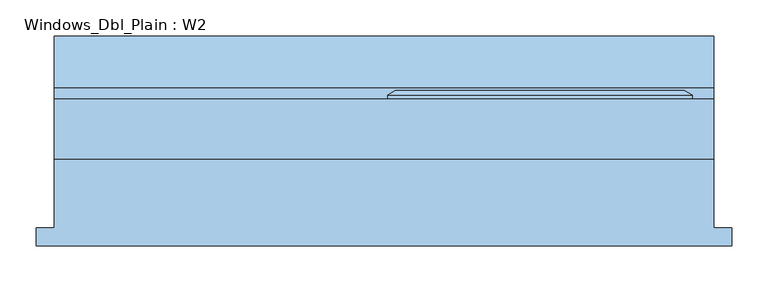
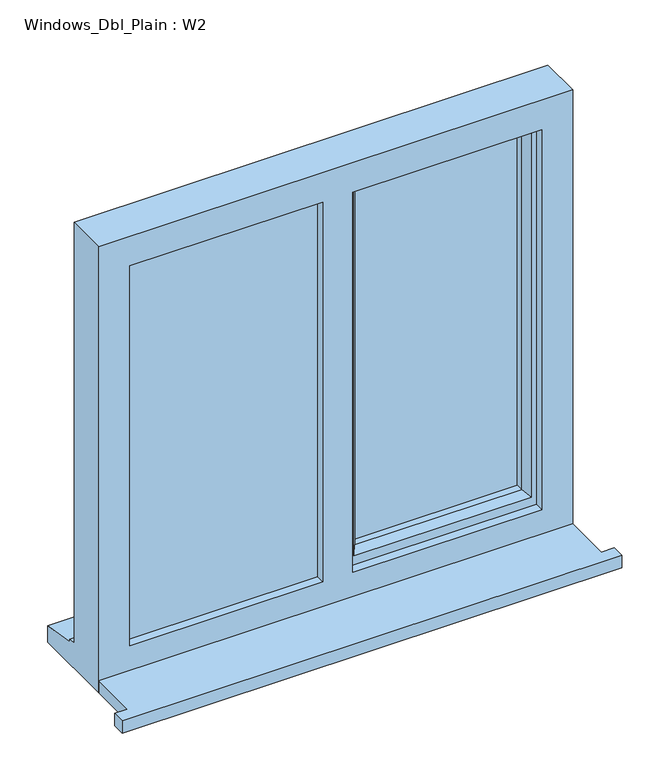
"""IFC4 building model written with IfcOpenShell, lengths in millimetres: window geometry, Windows_Dbl_Plain : W2."""

from ifc_helpers import new_model, si_unit, frame, origin, place, context, project, spatial, polyline, outline, extrude, faceted_brep, source, transform, mapped, element, save


def windows_dbl_plain_w2_c69f14ef(model_context):
    return source(origin(), model_context, "Body", "SolidModel", [
        extrude(outline(polyline([(-767.2, -130.8434322), (-767.2, -105.8434322), (-742.2, -105.8434322), (-742.2, -10.2434322), (172.2, -10.2434322), (172.2, -105.8434322), (197.2, -105.8434322), (197.2, -130.8434322), (-767.2, -130.8434322)])), frame((0.0, 0.0, 1200.0), z_axis=(0.0, 0.0, 1.0), x_axis=(1.0, 0.0, 0.0)), (0.0, 0.0, 1.0), 25.0),
        faceted_brep([(-280.0, 72.7565678, 2080.0), (-280.0, 78.5300705, 2080.0), (-280.0, 78.5300705, 1253.0), (-280.0, 72.7565678, 1253.0), (-270.0, 7.7565678, 2070.0), (-270.0, 72.7565678, 2070.0), (-270.0, 72.7565678, 1263.0), (-270.0, 7.7565678, 1263.0), (-230.0, 22.2494677, 2030.0), (-240.1480377, 7.7565678, 2040.1480377), (-240.1480377, 7.7565678, 1292.8519623), (-230.0, 22.2494677, 1303.0), (-230.0, 36.7565678, 2030.0), (-230.0, 36.7565678, 1303.0), (-240.0, 60.7565678, 2040.0), (-240.0, 36.7565678, 2040.0), (-240.0, 36.7565678, 1293.0), (-240.0, 60.7565678, 1293.0), (-230.0, 78.5300705, 2030.0), (-230.0, 60.7565678, 2030.0), (-230.0, 60.7565678, 1303.0), (-230.0, 78.5300705, 1303.0), (-247.4457548, 84.3035732, 2047.4457548), (-247.4457548, 84.3035732, 1285.5542452), (-269.2153903, 84.3035732, 2069.2153903), (-269.2153903, 84.3035732, 1263.7846097), (142.2, 78.5300705, 1253.0), (142.2, 72.7565678, 1253.0), (132.2, 72.7565678, 1263.0), (132.2, 7.7565678, 1263.0), (102.3480377, 7.7565678, 1292.8519623), (92.2, 22.2494677, 1303.0), (92.2, 36.7565678, 1303.0), (102.2, 36.7565678, 1293.0), (102.2, 60.7565678, 1293.0), (92.2, 60.7565678, 1303.0), (92.2, 78.5300705, 1303.0), (109.6457548, 84.3035732, 1285.5542452), (131.4153903, 84.3035732, 1263.7846097), (142.2, 78.5300705, 2080.0), (142.2, 72.7565678, 2080.0), (132.2, 72.7565678, 2070.0), (132.2, 7.7565678, 2070.0), (102.3480377, 7.7565678, 2040.1480377), (92.2, 22.2494677, 2030.0), (92.2, 36.7565678, 2030.0), (102.2, 36.7565678, 2040.0), (102.2, 60.7565678, 2040.0), (92.2, 60.7565678, 2030.0), (92.2, 78.5300705, 2030.0), (109.6457548, 84.3035732, 2047.4457548), (131.4153903, 84.3035732, 2069.2153903)], [[[0, 1, 2, 3]], [[4, 5, 6, 7]], [[8, 9, 10, 11]], [[12, 8, 11, 13]], [[14, 15, 16, 17]], [[18, 19, 20, 21]], [[22, 18, 21, 23]], [[1, 24, 25, 2]], [[3, 2, 26, 27]], [[7, 6, 28, 29]], [[11, 10, 30, 31]], [[13, 11, 31, 32]], [[17, 16, 33, 34]], [[21, 20, 35, 36]], [[23, 21, 36, 37]], [[2, 25, 38, 26]], [[27, 26, 39, 40]], [[29, 28, 41, 42]], [[31, 30, 43, 44]], [[32, 31, 44, 45]], [[34, 33, 46, 47]], [[36, 35, 48, 49]], [[37, 36, 49, 50]], [[26, 38, 51, 39]], [[40, 39, 1, 0]], [[3, 27, 40, 0], [5, 41, 28, 6]], [[42, 41, 5, 4]], [[7, 29, 42, 4], [9, 43, 30, 10]], [[44, 43, 9, 8]], [[45, 44, 8, 12]], [[15, 46, 33, 16], [13, 32, 45, 12]], [[47, 46, 15, 14]], [[17, 34, 47, 14], [19, 48, 35, 20]], [[49, 48, 19, 18]], [[50, 49, 18, 22]], [[24, 51, 38, 25], [23, 37, 50, 22]], [[39, 51, 24, 1]]]),
        extrude(outline(polyline([(2050.0, -310.0), (2070.0, -310.0), (2070.0, -702.2), (1263.0, -702.2), (1263.0, -310.0), (1283.0, -310.0), (1283.0, -682.2), (2050.0, -682.2), (2050.0, -310.0)])), frame((0.0, 31.7565678, 0.0), z_axis=(0.0, 1.0, 0.0), x_axis=(0.0, 0.0, 1.0)), (0.0, 0.0, 1.0), 41.0),
        faceted_brep([(172.2, -10.2434322, 2110.0), (-742.2, -10.2434322, 2110.0), (-742.2, -10.2434322, 1200.0), (172.2, -10.2434322, 1200.0), (112.2, -10.2434322, 2050.0), (112.2, -10.2434322, 1275.0), (-252.0, -10.2434322, 1275.0), (-252.0, -10.2434322, 2050.0), (-310.0, -10.2434322, 2050.0), (-310.0, -10.2434322, 1275.0), (-682.2, -10.2434322, 1275.0), (-682.2, -10.2434322, 2050.0), (-742.2, 72.7565678, 2110.0), (-742.2, 72.7565678, 1251.0), (-742.2, 87.7565678, 1249.68767), (-742.2, 87.7565678, 1244.7449676), (-742.2, 160.2565678, 1233.8088847), (-742.2, 160.2565678, 1200.0), (172.2, 72.7565678, 2110.0), (172.2, 72.7565678, 1251.0), (-702.2, 72.7565678, 2070.0), (-702.2, 72.7565678, 1263.0), (-310.0, 72.7565678, 1263.0), (-310.0, 72.7565678, 2070.0), (-270.0, 72.7565678, 2070.0), (-270.0, 72.7565678, 1263.0), (132.2, 72.7565678, 1263.0), (132.2, 72.7565678, 2070.0), (-702.2, 7.7565678, 2070.0), (-702.2, 7.7565678, 1263.0), (-300.0, 7.7565678, 2070.0), (-300.0, 7.7565678, 1263.0), (-310.0, 7.7565678, 2050.0), (-682.2, 7.7565678, 2050.0), (-682.2, 7.7565678, 1275.0), (-310.0, 7.7565678, 1275.0), (-270.0, 7.7565678, 2070.0), (132.2, 7.7565678, 2070.0), (132.2, 7.7565678, 1263.0), (-270.0, 7.7565678, 1263.0), (112.2, 7.7565678, 2050.0), (-252.0, 7.7565678, 2050.0), (-252.0, 7.7565678, 1275.0), (112.2, 7.7565678, 1275.0), (-310.0, 31.7565678, 2070.0), (-300.0, 31.7565678, 2070.0), (172.2, 160.2565678, 1200.0), (172.2, 160.2565678, 1233.8088847), (172.2, 87.7565678, 1244.7449676), (172.2, 87.7565678, 1249.68767), (-300.0, 31.7565678, 1263.0), (-310.0, 31.7565678, 1263.0)], [[[0, 1, 2, 3], [4, 5, 6, 7], [8, 9, 10, 11]], [[2, 1, 12, 13, 14, 15, 16, 17]], [[13, 12, 18, 19], [20, 21, 22, 23], [24, 25, 26, 27]], [[21, 20, 28, 29]], [[28, 30, 31, 29], [32, 33, 34, 35]], [[36, 37, 38, 39], [40, 41, 42, 43]], [[33, 11, 10, 34]], [[1, 0, 18, 12]], [[28, 20, 23, 44, 45, 30]], [[27, 37, 36, 24]], [[11, 33, 32, 8]], [[40, 4, 7, 41]], [[19, 18, 0, 3, 46, 47, 48, 49]], [[27, 26, 38, 37]], [[4, 40, 43, 5]], [[45, 50, 31, 30]], [[50, 45, 44, 51]], [[51, 44, 23, 22]], [[25, 24, 36, 39]], [[41, 7, 6, 42]], [[8, 32, 35, 9]], [[46, 3, 2, 17]], [[47, 46, 17, 16]], [[48, 47, 16, 15]], [[49, 48, 15, 14]], [[19, 49, 14, 13]], [[22, 21, 29, 31, 50, 51]], [[26, 25, 39, 38]], [[6, 5, 43, 42]], [[35, 34, 10, 9]]]),
        extrude(outline(polyline([(-702.2, 31.7565678), (-300.0, 31.7565678), (-300.0, 7.7565678), (-702.2, 7.7565678), (-702.2, 31.7565678)])), frame((0.0, 0.0, 1263.0), z_axis=(0.0, 0.0, 1.0), x_axis=(1.0, 0.0, 0.0)), (0.0, 0.0, 1.0), 807.0),
        extrude(outline(polyline([(102.2, 36.7565678), (-240.0, 36.7565678), (-240.0, 60.7565678), (102.2, 60.7565678), (102.2, 36.7565678)])), frame((0.0, 0.0, 1293.0), z_axis=(0.0, 0.0, 1.0), x_axis=(1.0, 0.0, 0.0)), (0.0, 0.0, 1.0), 747.0),
    ])


if __name__ == "__main__":
    model = new_model("IFC4")
    model_context = context("Model", 3, world=origin())
    ifc_project = project(units=[si_unit("LENGTHUNIT", "METRE", prefix="MILLI")], contexts=[model_context])
    site = spatial("IfcSite", under=ifc_project)
    building = spatial("IfcBuilding", under=site)
    placement = place(None, origin())
    windows_dbl_plain_w2_shape = windows_dbl_plain_w2_c69f14ef(model_context)
    element("IfcWindow", 1, ObjectType="Windows_Dbl_Plain : W2", at=placement, inside=building, context=model_context, shape_type="MappedRepresentation", body=[
        mapped(windows_dbl_plain_w2_shape, transform((0.0, 0.0, 0.0), x_axis=(1.0, 0.0, 0.0), y_axis=(0.0, 1.0, 0.0), z_axis=(0.0, 0.0, 1.0))),
    ])
    save(model, "model.ifc")

# Revit data of these elements
# Type "Windows_Dbl_Plain : W2"
#   Type Mark = "57"
#   Operation = "DoublePanelVertical"
#   Construction Type Id = "GSP4R"
#   Manufacturer = "Revit"
#   Keynote = "L10"
#   Analytic Construction = "1/8 in Pilkington single glazing"
#   Wrap Layers (Ext) from Ext = 0.336286 ft
#   Wrap Layers (Int) from Ext = 0.582349 ft
#   Window Board Projection = 0.082021 ft
#   Window Board Extension = 0.082021 ft
#   Visual Light Transmittance = 0.9
#   Solar Heat Gain Coefficient = 0.78
#   Rough Width = 3.0 ft
#   Rough Height = 2.985564 ft
#   Height = 2.985564 ft
#   Width = 3.0 ft
#   Heat Transfer Coefficient (U) = 3.6886 W/(m²·K)
#   Glazing Thickness = 0.07874 ft
#   FrameOffset - External = 0.164042 ft
#   Frame Depth = 0.213255 ft
#   Default Head Height = 6.922572 ft
#   Cill Depth = 0.287073 ft
#   Cavity Closer Width = 0.164042 ft
#   Cavity Closer Offset from Ext = 0.336286 ft
#   Cavity Closer Depth = 0.278871 ft
#   Vis - Cavity Closers = yes
#   Define Thermal Properties by = 1
#   Material Trim = Window Frame
#   Material Glass = Glass
#   Material Frame = Window Frame
#   Wall Closure = (empty or 0)
# Element 1 (IfcWindow, "Windows_Dbl_Plain : W2")
#   Materials on its faces: "Window Frame", "Glass"
# Materials
#   "Window Frame": colour RGB 249 249 249, transparency 0, Keynote = "L10", Cost = 0
#   "Glass": class "Glass", colour RGB 0 128 192, transparency 0.9, Description = "Soda Lime Glass", Cost = 0
